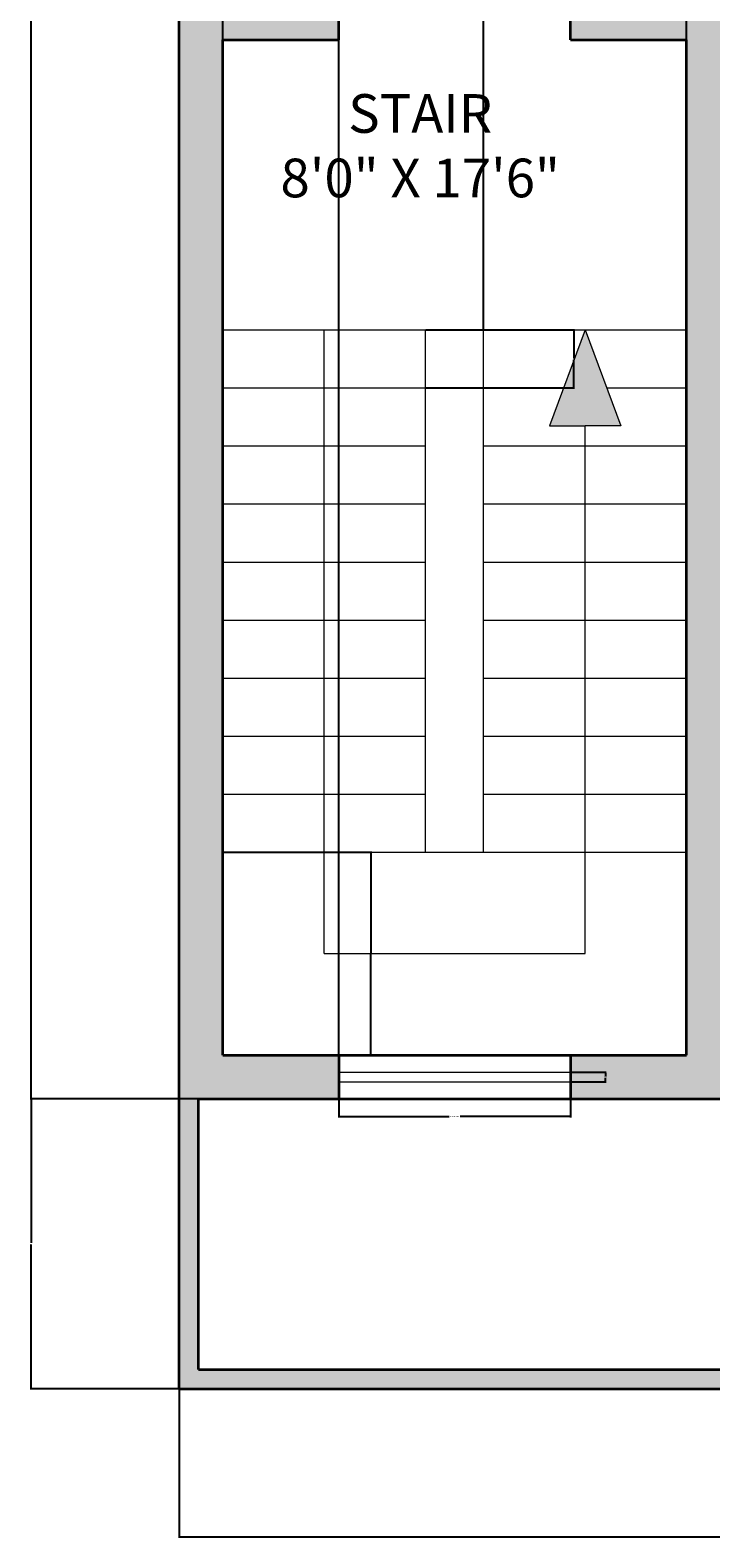
# Model space of a CAD drawing. Units: inches. Extents: x 1567 to 1964, y 1813 to 2447.
# Tile 1 of 28: x 1567 to 1707, y 1813 to 2125. Entities that reach past the tile are written whole.
import ezdxf

# ---------------------------------------------------------------- set-up
doc = ezdxf.new("R2010")
doc.units = ezdxf.units.IN
for name, color, linetype, lineweight in [('A-ANNO-DIMS', 2, 'Continuous', 18), ('A-AREA-IDEN', 7, 'Continuous', 18), ('A-FLOR-STRS', 7, 'Continuous', 18), ('A-GLAZ', 4, 'Continuous', 18), ('A-WALL', 7, 'Continuous', 35)]:
    doc.layers.add(name, color=color, linetype=linetype, lineweight=lineweight)
doc.layers.add('A-FURN-PATT', color=252, linetype='Continuous', lineweight=13, true_color=0x939598)
doc.layers.add('A-WALL-PATT', color=251, linetype='Continuous', lineweight=13, true_color=0x636466)
doc.styles.get("Standard").update_dxf_attribs({"font": 'arial.ttf'})
doc.dimstyles.get("Standard").update_dxf_attribs({"dimtxt": 0.18, "dimasz": 0.18, "dimexe": 0.18, "dimexo": 0.0625, "dimgap": 0.09, "dimtad": 0, "dimtih": 1, "dimtoh": 1, "dimdec": 4, "dimzin": 0, "dimdsep": 46, "dimtxsty": 'Standard', "dimcen": 0.09, "dimadec": 0, "dimazin": 0, "dimtfac": 1, "dimtdec": 4, "dimtofl": 0, "dimtmove": 0, "dimatfit": 3, "dimfxl": 1, "dimtolj": 1, "dimtzin": 0, "dimarcsym": 0})

# ---------------------------------------------------------------- blocks, each defined once
blk = doc.blocks.new('WINDOW-48IN')
for p, q in [((0, 2), (48, 2)), ((0, 0), (48, 0))]:
    blk.add_line(p, q)
blk = doc.blocks.new('*D35')
at = {"layer": 'A-ANNO-DIMS', "color": 0, "lineweight": -2, "transparency": 16777216}
for p, q in [((1630.43, 1907.73), (1630.43, 1900.41)), ((1678.43, 1907.73), (1678.43, 1900.41)), ((1630.61, 1900.59), (1653.31, 1900.59)), ((1678.25, 1900.59), (1655.55, 1900.59))]:
    blk.add_line(p, q, dxfattribs=at)
at = {"layer": 'A-ANNO-DIMS', "color": 0, "transparency": 16777216}
for points in [[(1630.61, 1900.62), (1630.61, 1900.56), (1630.43, 1900.59)], [(1678.25, 1900.62), (1678.25, 1900.56), (1678.43, 1900.59)]]:
    blk.add_solid(points, dxfattribs=at)
at = {"layer": 'Defpoints', "color": 0, "transparency": 16777216}
for p in [(1630.43, 1907.79), (1678.43, 1907.79), (1678.43, 1900.59)]:
    blk.add_point(p, dxfattribs=at)
at = {"layer": 'A-ANNO-DIMS', "color": 0, "transparency": 16777216, "insert": (1654.43, 1900.59), "char_height": 0.18, "attachment_point": 5}
blk.add_mtext('\\A1;WINDOW 48 TYP.', dxfattribs=at)
blk = doc.blocks.new('*D36')
at = {"layer": 'A-ANNO-DIMS', "color": 0, "lineweight": -2, "transparency": 16777216}
for p, q in [((1678.49, 1909.79), (1685.81, 1909.79)), ((1685.63, 1909.61), (1685.63, 1908.97)), ((1685.63, 1907.97), (1685.63, 1908.61)), ((1678.49, 1907.79), (1685.81, 1907.79))]:
    blk.add_line(p, q, dxfattribs=at)
at = {"layer": 'A-ANNO-DIMS', "color": 0, "transparency": 16777216}
for points in [[(1685.6, 1909.61), (1685.66, 1909.61), (1685.63, 1909.79)], [(1685.6, 1907.97), (1685.66, 1907.97), (1685.63, 1907.79)]]:
    blk.add_solid(points, dxfattribs=at)
at = {"layer": 'Defpoints', "color": 0, "transparency": 16777216}
for p in [(1678.43, 1909.79), (1685.63, 1909.79), (1678.43, 1907.79)]:
    blk.add_point(p, dxfattribs=at)
at = {"layer": 'A-ANNO-DIMS', "color": 0, "transparency": 16777216, "insert": (1685.63, 1908.79), "char_height": 0.18, "attachment_point": 5}
blk.add_mtext('\\A1;2 TYP.', dxfattribs=at)
blk = doc.blocks.new('*D39')
at = {"layer": 'A-ANNO-DIMS', "color": 0, "lineweight": -2, "transparency": 16777216}
for p, q in [((1597.43, 1844.23), (1597.43, 1813.46)), ((1933.43, 1844.23), (1933.43, 1813.46)), ((1597.61, 1813.64), (1765.14, 1813.64)), ((1933.25, 1813.64), (1765.72, 1813.64))]:
    blk.add_line(p, q, dxfattribs=at)
at = {"layer": 'A-ANNO-DIMS', "color": 0, "transparency": 16777216}
for points in [[(1597.61, 1813.67), (1597.61, 1813.61), (1597.43, 1813.64)], [(1933.25, 1813.67), (1933.25, 1813.61), (1933.43, 1813.64)]]:
    blk.add_solid(points, dxfattribs=at)
at = {"layer": 'Defpoints', "color": 0, "transparency": 16777216}
for p in [(1597.43, 1844.29), (1933.43, 1844.29), (1933.43, 1813.64)]:
    blk.add_point(p, dxfattribs=at)
at = {"layer": 'A-ANNO-DIMS', "color": 0, "transparency": 16777216, "insert": (1765.43, 1813.64), "char_height": 0.18, "attachment_point": 5}
blk.add_mtext('\\A1;336', dxfattribs=at)
blk = doc.blocks.new('*D41')
at = {"layer": 'A-ANNO-DIMS', "color": 0, "lineweight": -2, "transparency": 16777216}
for p, q in [((1597.37, 2416.29), (1566.6, 2416.29)), ((1566.78, 2416.11), (1566.78, 2160.47)), ((1566.78, 1904.47), (1566.78, 2160.11)), ((1601.37, 1904.29), (1566.6, 1904.29))]:
    blk.add_line(p, q, dxfattribs=at)
at = {"layer": 'A-ANNO-DIMS', "color": 0, "transparency": 16777216}
for points in [[(1566.75, 2416.11), (1566.81, 2416.11), (1566.78, 2416.29)], [(1566.75, 1904.47), (1566.81, 1904.47), (1566.78, 1904.29)]]:
    blk.add_solid(points, dxfattribs=at)
at = {"layer": 'Defpoints', "color": 0, "transparency": 16777216}
for p in [(1566.78, 2416.29), (1597.43, 2416.29), (1601.43, 1904.29)]:
    blk.add_point(p, dxfattribs=at)
at = {"layer": 'A-ANNO-DIMS', "color": 0, "transparency": 16777216, "insert": (1566.78, 2160.29), "char_height": 0.18, "attachment_point": 5}
blk.add_mtext('\\A1;512', dxfattribs=at)
blk = doc.blocks.new('*D42')
at = {"layer": 'A-ANNO-DIMS', "color": 0, "lineweight": -2, "transparency": 16777216}
for p, q in [((1601.37, 1904.29), (1566.6, 1904.29)), ((1566.78, 1904.11), (1566.78, 1874.47)), ((1566.78, 1844.47), (1566.78, 1874.11)), ((1597.37, 1844.29), (1566.6, 1844.29))]:
    blk.add_line(p, q, dxfattribs=at)
at = {"layer": 'A-ANNO-DIMS', "color": 0, "transparency": 16777216}
for points in [[(1566.75, 1904.11), (1566.81, 1904.11), (1566.78, 1904.29)], [(1566.75, 1844.47), (1566.81, 1844.47), (1566.78, 1844.29)]]:
    blk.add_solid(points, dxfattribs=at)
at = {"layer": 'Defpoints', "color": 0, "transparency": 16777216}
for p in [(1566.78, 1904.29), (1601.43, 1904.29), (1597.43, 1844.29)]:
    blk.add_point(p, dxfattribs=at)
at = {"layer": 'A-ANNO-DIMS', "color": 0, "transparency": 16777216, "insert": (1566.78, 1874.29), "char_height": 0.18, "attachment_point": 5}
blk.add_mtext('\\A1;60', dxfattribs=at)
blk = doc.blocks.new('*D53')
at = {"layer": 'A-ANNO-DIMS', "color": 0, "lineweight": -2, "transparency": 16777216}
for p, q in [((1606.43, 1913.35), (1606.43, 2447.12)), ((1606.61, 2446.94), (1618.21, 2446.94)), ((1630.25, 2446.94), (1618.65, 2446.94)), ((1630.43, 1913.35), (1630.43, 2447.12))]:
    blk.add_line(p, q, dxfattribs=at)
at = {"layer": 'A-ANNO-DIMS', "color": 0, "transparency": 16777216}
for points in [[(1606.61, 2446.97), (1606.61, 2446.91), (1606.43, 2446.94)], [(1630.25, 2446.97), (1630.25, 2446.91), (1630.43, 2446.94)]]:
    blk.add_solid(points, dxfattribs=at)
at = {"layer": 'Defpoints', "color": 0, "transparency": 16777216}
for p in [(1630.43, 2446.94), (1606.43, 1913.29), (1630.43, 1913.29)]:
    blk.add_point(p, dxfattribs=at)
at = {"layer": 'A-ANNO-DIMS', "color": 0, "transparency": 16777216, "insert": (1618.43, 2446.94), "char_height": 0.18, "attachment_point": 5}
blk.add_mtext('\\A1;24', dxfattribs=at)
blk = doc.blocks.new('*D60')
at = {"layer": 'A-ANNO-DIMS', "color": 0, "lineweight": -2, "transparency": 16777216}
for p, q in [((1660.43, 2063.35), (1660.43, 2447.12)), ((1660.61, 2446.94), (1681.21, 2446.94)), ((1702.25, 2446.94), (1681.65, 2446.94)), ((1702.43, 2063.35), (1702.43, 2447.12))]:
    blk.add_line(p, q, dxfattribs=at)
at = {"layer": 'A-ANNO-DIMS', "color": 0, "transparency": 16777216}
for points in [[(1660.61, 2446.97), (1660.61, 2446.91), (1660.43, 2446.94)], [(1702.25, 2446.97), (1702.25, 2446.91), (1702.43, 2446.94)]]:
    blk.add_solid(points, dxfattribs=at)
at = {"layer": 'Defpoints', "color": 0, "transparency": 16777216}
for p in [(1660.43, 2446.94), (1660.43, 2063.29), (1702.43, 2063.29)]:
    blk.add_point(p, dxfattribs=at)
at = {"layer": 'A-ANNO-DIMS', "color": 0, "transparency": 16777216, "insert": (1681.43, 2446.94), "char_height": 0.18, "attachment_point": 5}
blk.add_mtext('\\A1;42', dxfattribs=at)
blk = doc.blocks.new('*D61')
at = {"layer": 'A-ANNO-DIMS', "color": 0, "lineweight": -2, "transparency": 16777216}
for p, q in [((1648.49, 2063.29), (1679.26, 2063.29)), ((1679.08, 2063.11), (1679.08, 2057.47)), ((1679.08, 2051.47), (1679.08, 2057.11)), ((1648.49, 2051.29), (1679.26, 2051.29))]:
    blk.add_line(p, q, dxfattribs=at)
at = {"layer": 'A-ANNO-DIMS', "color": 0, "transparency": 16777216}
for points in [[(1679.05, 2063.11), (1679.11, 2063.11), (1679.08, 2063.29)], [(1679.05, 2051.47), (1679.11, 2051.47), (1679.08, 2051.29)]]:
    blk.add_solid(points, dxfattribs=at)
at = {"layer": 'Defpoints', "color": 0, "transparency": 16777216}
for p in [(1648.43, 2063.29), (1648.43, 2051.29), (1679.08, 2051.29)]:
    blk.add_point(p, dxfattribs=at)
at = {"layer": 'A-ANNO-DIMS', "color": 0, "transparency": 16777216, "insert": (1679.08, 2057.29), "char_height": 0.18, "attachment_point": 5}
blk.add_mtext('\\A1;12', dxfattribs=at)
blk = doc.blocks.new('*D62')
at = {"layer": 'A-ANNO-DIMS', "color": 0, "lineweight": -2, "transparency": 16777216}
for p, q in [((1606.49, 1955.29), (1637.26, 1955.29)), ((1637.08, 1955.11), (1637.08, 1934.47)), ((1637.08, 1913.47), (1637.08, 1934.11)), ((1606.49, 1913.29), (1637.26, 1913.29))]:
    blk.add_line(p, q, dxfattribs=at)
at = {"layer": 'A-ANNO-DIMS', "color": 0, "transparency": 16777216}
for points in [[(1637.05, 1955.11), (1637.11, 1955.11), (1637.08, 1955.29)], [(1637.05, 1913.47), (1637.11, 1913.47), (1637.08, 1913.29)]]:
    blk.add_solid(points, dxfattribs=at)
at = {"layer": 'Defpoints', "color": 0, "transparency": 16777216}
for p in [(1606.43, 1955.29), (1606.43, 1913.29), (1637.08, 1913.29)]:
    blk.add_point(p, dxfattribs=at)
at = {"layer": 'A-ANNO-DIMS', "color": 0, "transparency": 16777216, "insert": (1637.08, 1934.29), "char_height": 0.18, "attachment_point": 5}
blk.add_mtext('\\A1;42', dxfattribs=at)

msp = doc.modelspace()

# ---------------------------------------------------------------- hatches: boundary and pattern name
at = {"layer": 'A-FURN-PATT'}
h = msp.add_hatch(color=256, dxfattribs=at)
h.dxf.hatch_style = 1
h.paths.add_polyline_path([(1697.3402, 2374.8316), (1682.1402, 2374.8316), (1682.1402, 2387.6316), (1637.3402, 2387.6316), (1637.3402, 2324.4315), (1697.3402, 2324.4315)])
h.paths.add_polyline_path([(1891.1093, 2375.8204), (1875.9094, 2375.8204), (1875.9094, 2388.6204), (1831.1094, 2388.6204), (1831.1094, 2325.4204), (1891.1093, 2325.4204)])
h.paths.add_polyline_path([(1702.5611, 2206.8057), (1702.5611, 2210.8057), (1699.7395, 2209.9436), (1697.013, 2209.2403), (1694.3857, 2208.6763), (1691.8615, 2208.2326), (1689.4443, 2207.8896), (1687.1381, 2207.6282), (1684.9469, 2207.4289), (1682.8747, 2207.2725), (1680.9233, 2207.1425), (1679.0865, 2207.0339), (1677.3558, 2206.9445), (1675.7229, 2206.8719), (1674.1794, 2206.8141), (1672.7169, 2206.7688), (1671.327, 2206.7339), (1670.0014, 2206.707), (1668.7314, 2206.6866), (1667.5072, 2206.6732), (1666.3188, 2206.668), (1665.1561, 2206.6722), (1664.009, 2206.6869), (1662.8675, 2206.7133), (1661.7215, 2206.7525), (1660.5611, 2206.8057), (1660.5611, 2202.8057), (1661.9932, 2202.9556), (1663.3314, 2203.0744), (1664.5899, 2203.1671), (1665.7831, 2203.2385), (1666.9254, 2203.2935), (1668.0311, 2203.3368), (1669.1145, 2203.3734), (1670.1902, 2203.4081), (1671.2724, 2203.4451), (1672.3759, 2203.4866), (1673.5155, 2203.534), (1674.706, 2203.5887), (1675.9621, 2203.6523), (1677.2986, 2203.7262), (1678.7304, 2203.8118), (1680.2722, 2203.9108), (1681.947, 2204.0272), (1683.8108, 2204.1769), (1685.9279, 2204.3782), (1688.3626, 2204.6496), (1691.179, 2205.0096), (1694.4413, 2205.4767), (1698.214, 2206.0692)])
h.paths.add_polyline_path([(1702.5611, 2218.8057), (1701.9821, 2217.9383), (1701.3316, 2217.191), (1700.6091, 2216.5515), (1699.8141, 2216.0071), (1698.946, 2215.5454), (1698.0041, 2215.1536), (1696.9879, 2214.8194), (1695.8969, 2214.5301), (1694.7328, 2214.2753), (1693.5072, 2214.0522), (1692.2339, 2213.8602), (1690.9266, 2213.6989), (1689.5994, 2213.5675), (1688.266, 2213.4654), (1686.9402, 2213.392), (1685.636, 2213.3467), (1684.3619, 2213.3287), (1683.1053, 2213.3361), (1681.8482, 2213.3668), (1680.5727, 2213.4187), (1679.2608, 2213.4898), (1677.8948, 2213.5779), (1676.4565, 2213.6811), (1674.9282, 2213.7971), (1673.2982, 2213.9236), (1671.5804, 2214.0573), (1669.795, 2214.1945), (1667.9622, 2214.3316), (1666.1022, 2214.4649), (1664.2352, 2214.5908), (1662.3814, 2214.7056), (1660.5611, 2214.8057), (1660.5611, 2206.8057), (1661.7215, 2206.7525), (1662.8675, 2206.7133), (1664.009, 2206.6869), (1665.1561, 2206.6722), (1666.3188, 2206.668), (1667.5072, 2206.6732), (1668.7314, 2206.6866), (1670.0014, 2206.707), (1671.327, 2206.7339), (1672.7169, 2206.7688), (1674.1794, 2206.8141), (1675.7229, 2206.8719), (1677.3558, 2206.9445), (1679.0865, 2207.0339), (1680.9233, 2207.1425), (1682.8747, 2207.2725), (1684.9469, 2207.4289), (1687.1381, 2207.6282), (1689.4443, 2207.8896), (1691.8615, 2208.2326), (1694.3857, 2208.6763), (1697.013, 2209.2403), (1699.7395, 2209.9436), (1702.5611, 2210.8057)])
h.paths.add_polyline_path([(1700.6091, 2216.5515), (1701.3316, 2217.191), (1701.9821, 2217.9383), (1702.5611, 2218.8057), (1702.5611, 2222.8057), (1689.452, 2222.8057), (1689.0171, 2222.4556), (1688.4521, 2222.0354), (1687.7806, 2221.5662), (1687.0235, 2221.067), (1686.2019, 2220.5566), (1685.3367, 2220.0541), (1684.4491, 2219.5785), (1683.56, 2219.1486), (1682.6867, 2218.7795), (1681.8312, 2218.4692), (1680.9918, 2218.212), (1680.1667, 2218.0019), (1679.3541, 2217.833), (1678.5524, 2217.6995), (1677.7597, 2217.5954), (1676.9744, 2217.5149), (1676.1942, 2217.4531), (1675.4146, 2217.4093), (1674.6309, 2217.384), (1673.8381, 2217.3774), (1673.0313, 2217.39), (1672.2056, 2217.4221), (1671.3562, 2217.4741), (1670.4782, 2217.5463), (1669.5642, 2217.639), (1668.5968, 2217.7516), (1667.5562, 2217.8833), (1666.4226, 2218.0336), (1665.1761, 2218.2017), (1663.7969, 2218.3869), (1662.2651, 2218.5885), (1660.5611, 2218.8057), (1660.5611, 2214.8057), (1662.3814, 2214.7056), (1664.2352, 2214.5908), (1666.1022, 2214.4649), (1667.9622, 2214.3316), (1669.795, 2214.1945), (1671.5804, 2214.0573), (1673.2982, 2213.9236), (1674.9282, 2213.7971), (1676.4565, 2213.6811), (1677.8948, 2213.5779), (1679.2608, 2213.4898), (1680.5727, 2213.4187), (1681.8482, 2213.3668), (1683.1053, 2213.3361), (1684.3619, 2213.3287), (1685.636, 2213.3467), (1686.9402, 2213.392), (1688.266, 2213.4654), (1689.5994, 2213.5675), (1690.9266, 2213.6989), (1692.2339, 2213.8602), (1693.5072, 2214.0522), (1694.7328, 2214.2753), (1695.8969, 2214.5301), (1696.9879, 2214.8194), (1698.0041, 2215.1536), (1698.946, 2215.5454), (1699.8141, 2216.0071)])
h.paths.add_polyline_path([(1687.0235, 2221.067), (1687.7806, 2221.5662), (1688.4521, 2222.0354), (1689.0171, 2222.4556), (1689.452, 2222.8057), (1660.5611, 2222.8057), (1660.5611, 2218.8057), (1662.2651, 2218.5885), (1663.7969, 2218.3869), (1665.1761, 2218.2017), (1666.4226, 2218.0336), (1667.5562, 2217.8833), (1668.5968, 2217.7516), (1669.5642, 2217.639), (1670.4782, 2217.5463), (1671.3562, 2217.4741), (1672.2056, 2217.4221), (1673.0313, 2217.39), (1673.8381, 2217.3774), (1674.6309, 2217.384), (1675.4146, 2217.4093), (1676.1942, 2217.4531), (1676.9744, 2217.5149), (1677.7597, 2217.5954), (1678.5524, 2217.6995), (1679.3541, 2217.833), (1680.1667, 2218.0019), (1680.9918, 2218.212), (1681.8312, 2218.4692), (1682.6867, 2218.7795), (1683.56, 2219.1486), (1684.4491, 2219.5785), (1685.3367, 2220.0541), (1686.2019, 2220.5566)], flags=17)
h.paths.add_polyline_path([(1702.5611, 2198.8057), (1698.9289, 2199.2412), (1695.8472, 2199.5774), (1693.2166, 2199.8257), (1690.9377, 2199.9973), (1688.9111, 2200.1033), (1687.0375, 2200.155), (1685.2174, 2200.1637), (1683.3514, 2200.1406), (1681.3514, 2200.0941), (1679.1736, 2200.0225), (1676.7858, 2199.921), (1674.1554, 2199.7852), (1671.2502, 2199.6103), (1668.0377, 2199.3919), (1664.4854, 2199.1252), (1660.5611, 2198.8057), (1660.5611, 2194.8057), (1662.2697, 2194.9771), (1663.9673, 2195.0999), (1665.6339, 2195.1809), (1667.2495, 2195.227), (1668.7941, 2195.2449), (1670.2478, 2195.2414), (1671.5906, 2195.2233), (1672.8026, 2195.1974), (1673.8739, 2195.1689), (1674.8359, 2195.1364), (1675.7302, 2195.0967), (1676.5982, 2195.0469), (1677.4817, 2194.9838), (1678.422, 2194.9043), (1679.4609, 2194.8055), (1680.6397, 2194.6842), (1682.005, 2194.5341), (1683.6223, 2194.335), (1685.562, 2194.0637), (1687.8945, 2193.6967), (1690.6902, 2193.2108), (1694.0196, 2192.5826), (1697.9531, 2191.7887), (1702.5611, 2190.8057)])
h.paths.add_polyline_path([(1702.5611, 2206.8057), (1698.214, 2206.0692), (1694.4413, 2205.4767), (1691.179, 2205.0096), (1688.3626, 2204.6496), (1685.9279, 2204.3782), (1683.8108, 2204.1769), (1681.947, 2204.0272), (1680.2722, 2203.9108), (1678.7304, 2203.8118), (1677.2986, 2203.7262), (1675.9621, 2203.6523), (1674.706, 2203.5887), (1673.5155, 2203.534), (1672.3759, 2203.4866), (1671.2724, 2203.4451), (1670.1902, 2203.4081), (1669.1145, 2203.3734), (1668.0311, 2203.3368), (1666.9254, 2203.2935), (1665.7831, 2203.2385), (1664.5899, 2203.1671), (1663.3314, 2203.0744), (1661.9932, 2202.9556), (1660.5611, 2202.8057), (1660.5611, 2198.8057), (1664.4854, 2199.1252), (1668.0377, 2199.3919), (1671.2502, 2199.6103), (1674.1554, 2199.7852), (1676.7858, 2199.921), (1679.1736, 2200.0225), (1681.3514, 2200.0941), (1683.3514, 2200.1406), (1685.2174, 2200.1637), (1687.0375, 2200.155), (1688.9111, 2200.1033), (1690.9377, 2199.9973), (1693.2166, 2199.8257), (1695.8472, 2199.5774), (1698.9289, 2199.2412), (1702.5611, 2198.8057)])
h.paths.add_polyline_path([(1702.5611, 2190.8057), (1697.9531, 2191.7887), (1694.0196, 2192.5826), (1690.6902, 2193.2108), (1687.8945, 2193.6967), (1685.562, 2194.0637), (1683.6223, 2194.335), (1682.005, 2194.5341), (1680.6397, 2194.6842), (1679.4609, 2194.8055), (1678.422, 2194.9043), (1677.4817, 2194.9838), (1676.5982, 2195.0469), (1675.7302, 2195.0967), (1674.8359, 2195.1364), (1673.8739, 2195.1689), (1672.8026, 2195.1974), (1671.5906, 2195.2233), (1670.2478, 2195.2414), (1668.7941, 2195.2449), (1667.2495, 2195.227), (1665.6339, 2195.1809), (1663.9673, 2195.0999), (1662.2697, 2194.9771), (1660.5611, 2194.8057), (1660.5611, 2190.8057), (1665.9637, 2190.2699), (1670.5105, 2189.7867), (1674.3035, 2189.3504), (1677.4445, 2188.9552), (1680.0354, 2188.5951), (1682.1782, 2188.2644), (1683.9747, 2187.9571), (1685.5268, 2187.6675), (1686.9225, 2187.3901), (1688.1943, 2187.1216), (1689.3606, 2186.859), (1690.4399, 2186.5993), (1691.4508, 2186.3396), (1692.4118, 2186.0769), (1693.3413, 2185.8084), (1694.2579, 2185.531), (1695.1786, 2185.2422), (1696.1142, 2184.9406), (1697.0739, 2184.6252), (1698.0671, 2184.2949), (1699.1032, 2183.9489), (1700.1913, 2183.586), (1701.3408, 2183.2053), (1702.5611, 2182.8057)])
h.paths.add_polyline_path([(1702.5611, 2182.8057), (1701.3408, 2183.2053), (1700.1913, 2183.586), (1699.1032, 2183.9489), (1698.0671, 2184.2949), (1697.0739, 2184.6252), (1696.1142, 2184.9406), (1695.1786, 2185.2422), (1694.2579, 2185.531), (1693.3413, 2185.8084), (1692.4118, 2186.0769), (1691.4508, 2186.3396), (1690.4399, 2186.5993), (1689.3606, 2186.859), (1688.1943, 2187.1216), (1686.9225, 2187.3901), (1685.5268, 2187.6675), (1683.9747, 2187.9571), (1682.1782, 2188.2644), (1680.0354, 2188.5951), (1677.4445, 2188.9552), (1674.3035, 2189.3504), (1670.5105, 2189.7867), (1665.9637, 2190.2699), (1660.5611, 2190.8057), (1660.5611, 2186.8057), (1663.5709, 2186.52), (1666.0965, 2186.2414), (1668.1979, 2185.9698), (1669.9351, 2185.7048), (1671.3681, 2185.446), (1672.5568, 2185.1931), (1673.5613, 2184.9458), (1674.4415, 2184.7037), (1675.2485, 2184.4664), (1675.9976, 2184.2328), (1677.0295, 2183.8907), (1678.2492, 2183.4332), (1679.354, 2182.9669), (1680.4123, 2182.4724), (1681.3757, 2181.9718), (1682.2435, 2181.4594), (1683.1864, 2180.8057), (1702.5611, 2180.8057)])
h.paths.add_polyline_path([(1677.3469, 2183.7716), (1676.6949, 2184.0016), (1675.9976, 2184.2328), (1675.2485, 2184.4664), (1674.4415, 2184.7037), (1673.5613, 2184.9458), (1672.5568, 2185.1931), (1671.3681, 2185.446), (1669.9351, 2185.7048), (1668.1979, 2185.9698), (1666.0965, 2186.2414), (1663.5709, 2186.52), (1660.5611, 2186.8057), (1660.5611, 2180.8057), (1683.1506, 2180.8057), (1682.802, 2181.0722), (1682.4264, 2181.3326), (1682.0201, 2181.5913), (1681.586, 2181.8476), (1681.1268, 2182.1011), (1680.6453, 2182.3513), (1680.1443, 2182.5976), (1679.6266, 2182.8395), (1679.0933, 2183.0769), (1678.5398, 2183.3105), (1677.9598, 2183.5417)], flags=17)
h.paths.add_polyline_path([(1824.4511, 2199.9016), (1824.089, 2199.9302), (1824.0595, 2199.9372), (1824.0397, 2199.9406), (1823.5413, 2200.0576), (1823.4095, 2200.0864), (1823.0664, 2200.1559), (1822.6419, 2200.2361), (1822.1519, 2200.3222), (1821.6126, 2200.4093), (1821.0401, 2200.4925), (1820.4505, 2200.5669), (1819.8599, 2200.6276), (1819.2845, 2200.6697), (1818.7366, 2200.6896), (1818.2141, 2200.688), (1817.7112, 2200.6668), (1817.222, 2200.6281), (1816.7405, 2200.5737), (1816.261, 2200.5057), (1815.7776, 2200.4259), (1815.2845, 2200.3364), (1814.3007, 2200.149), (1813.3315, 2199.9765), (1812.406, 2199.8514), (1811.6868, 2199.7739), (1810.8992, 2199.7121), (1810.0345, 2199.6697), (1809.0854, 2199.6497), (1808.0514, 2199.6502), (1806.9334, 2199.6683), (1805.7324, 2199.701), (1804.4493, 2199.7454), (1803.0852, 2199.7986), (1801.641, 2199.8577), (1800.1178, 2199.9197), (1798.5134, 2199.9818), (1796.8144, 2200.0415), (1795.004, 2200.0962), (1793.0657, 2200.1437), (1790.9828, 2200.1814), (1788.7389, 2200.2068), (1786.3171, 2200.2177), (1783.7011, 2200.2114), (1780.8715, 2200.185), (1777.7988, 2200.1326), (1774.4506, 2200.0481), (1770.7948, 2199.9249), (1766.7992, 2199.7569), (1762.4316, 2199.5376), (1757.6596, 2199.2606), (1752.4511, 2198.9197), (1752.4511, 2193.4197), (1761.2668, 2193.6071), (1768.3671, 2193.7934), (1773.9821, 2193.9778), (1778.3417, 2194.1593), (1781.6759, 2194.3369), (1784.2148, 2194.5096), (1786.1882, 2194.6764), (1787.8261, 2194.8364), (1789.3219, 2194.9887), (1790.7226, 2195.1333), (1792.0383, 2195.27), (1793.2792, 2195.3989), (1794.4557, 2195.52), (1795.5781, 2195.6333), (1796.6564, 2195.7387), (1797.7011, 2195.8364), (1798.7216, 2195.9259), (1799.7245, 2196.0057), (1800.7158, 2196.0737), (1801.7011, 2196.1281), (1802.6865, 2196.1668), (1803.6777, 2196.188), (1804.6806, 2196.1896), (1805.7011, 2196.1697), (1806.7423, 2196.1273), (1807.7962, 2196.0643), (1808.852, 2195.9837), (1809.899, 2195.8885), (1810.9265, 2195.7815), (1811.9238, 2195.6658), (1812.88, 2195.5442), (1813.7845, 2195.4197), (1814.6296, 2195.2948), (1815.4205, 2195.1704), (1816.1656, 2195.0469), (1816.873, 2194.9249), (1817.5511, 2194.8049), (1818.2083, 2194.6873), (1818.8527, 2194.5726), (1819.4928, 2194.4614), (1820.1348, 2194.3554), (1820.7773, 2194.2615), (1821.4169, 2194.1882), (1822.0501, 2194.1437), (1822.6735, 2194.1363), (1823.2838, 2194.1743), (1823.8775, 2194.266), (1824.4511, 2194.4197)])
h.paths.add_polyline_path([(1821.4716, 2190.5098), (1820.4303, 2190.5708), (1819.3811, 2190.6415), (1818.3339, 2190.7186), (1817.2985, 2190.7986), (1816.2845, 2190.8781), (1815.2976, 2190.9542), (1814.3274, 2191.0259), (1813.3592, 2191.0927), (1812.3782, 2191.1541), (1811.3699, 2191.2097), (1810.3196, 2191.2589), (1809.2127, 2191.3013), (1808.0345, 2191.3364), (1806.7708, 2191.3634), (1805.4094, 2191.3807), (1803.9387, 2191.3862), (1802.3469, 2191.3781), (1800.6223, 2191.3543), (1798.7532, 2191.313), (1796.7278, 2191.2521), (1794.5344, 2191.1697), (1792.128, 2191.0648), (1789.33, 2190.9393), (1785.9285, 2190.7962), (1781.7115, 2190.6385), (1776.4672, 2190.469), (1769.9836, 2190.2908), (1762.0489, 2190.1067), (1752.4511, 2189.9197), (1752.4511, 2185.4197), (1758.363, 2185.5846), (1763.4179, 2185.7075), (1767.7199, 2185.7933), (1771.373, 2185.8468), (1774.4811, 2185.873), (1777.1484, 2185.8768), (1779.4787, 2185.8629), (1781.5761, 2185.8364), (1783.5287, 2185.8014), (1785.3606, 2185.7596), (1787.0802, 2185.7119), (1788.6959, 2185.6593), (1790.2158, 2185.6028), (1791.6484, 2185.5434), (1793.0018, 2185.4821), (1794.2844, 2185.4197), (1795.5065, 2185.3576), (1796.6861, 2185.298), (1797.8433, 2185.2432), (1798.998, 2185.1958), (1800.1703, 2185.1581), (1801.3801, 2185.1326), (1802.6476, 2185.1218), (1803.9928, 2185.1281), (1805.4444, 2185.1555), (1807.0663, 2185.2147), (1808.9315, 2185.3178), (1811.1126, 2185.477), (1813.6823, 2185.7046), (1816.7135, 2186.0128), (1820.2788, 2186.4138), (1824.4511, 2186.9197), (1824.4511, 2190.4197), (1823.4918, 2190.4309), (1822.4954, 2190.4621)])
h.paths.add_polyline_path([(1797.3762, 2216.0584), (1797.6199, 2216.2267), (1797.9558, 2216.3355), (1798.3017, 2216.3703), (1798.5761, 2216.3781), (1798.8974, 2216.3703), (1799.2714, 2216.3468), (1799.704, 2216.3078), (1800.2011, 2216.2531), (1800.7695, 2216.1829), (1801.4205, 2216.0981), (1802.1662, 2215.9996), (1803.0188, 2215.8885), (1803.9906, 2215.7656), (1805.0937, 2215.632), (1806.3404, 2215.4886), (1807.7428, 2215.3364), (1809.3101, 2215.1764), (1811.039, 2215.0096), (1812.9232, 2214.8369), (1814.9563, 2214.6593), (1817.132, 2214.4778), (1819.444, 2214.2934), (1821.8858, 2214.1071), (1824.4511, 2213.9197), (1824.4511, 2217.9197), (1752.4511, 2217.9197), (1752.4511, 2214.9197), (1757.2739, 2214.8973), (1761.6432, 2214.8338), (1765.5973, 2214.7352), (1769.1751, 2214.6072), (1772.4149, 2214.4559), (1775.3554, 2214.2869), (1778.0352, 2214.1063), (1780.4928, 2213.9197), (1782.7607, 2213.7329), (1784.8476, 2213.5499), (1786.7557, 2213.3748), (1788.4876, 2213.2114), (1790.0456, 2213.0636), (1791.4322, 2212.9354), (1792.6499, 2212.8305), (1793.7011, 2212.7531), (1794.5904, 2212.7059), (1795.3313, 2212.688), (1795.9394, 2212.6974), (1796.4303, 2212.7322), (1796.8196, 2212.7905), (1797.123, 2212.8703), (1797.356, 2212.9695), (1797.5344, 2213.0864), (1797.6716, 2213.2187), (1797.7727, 2213.3637), (1797.8406, 2213.5185), (1797.8782, 2213.6801), (1797.8884, 2213.8457), (1797.8743, 2214.0122), (1797.8386, 2214.1767), (1797.7844, 2214.3364), (1797.7149, 2214.4889), (1797.6347, 2214.6346), (1797.5486, 2214.7744), (1797.3327, 2215.109), (1797.178, 2215.4303), (1797.1896, 2215.7939)])
h.paths.add_polyline_path([(1804.7872, 2210.6789), (1804.546, 2211.022), (1804.3512, 2211.3917), (1804.2466, 2211.7546), (1804.2574, 2212.0998), (1804.4058, 2212.4178), (1804.7068, 2212.7007), (1805.1359, 2212.9124), (1805.5279, 2212.9926), (1805.8136, 2213.0154), (1806.1178, 2213.0031), (1806.4405, 2212.9529), (1806.7929, 2212.867), (1807.1893, 2212.7489), (1807.6438, 2212.602), (1808.1706, 2212.4297), (1808.7838, 2212.2355), (1809.4976, 2212.0227), (1810.3261, 2211.7947), (1811.2868, 2211.5533), (1812.4101, 2211.2928), (1813.7297, 2211.0059), (1815.2793, 2210.6854), (1817.0925, 2210.3238), (1819.2031, 2209.9139), (1821.6447, 2209.4483), (1824.4511, 2208.9197), (1824.4511, 2213.9197), (1821.8858, 2214.1071), (1819.444, 2214.2934), (1817.132, 2214.4778), (1814.9563, 2214.6593), (1812.9232, 2214.8369), (1811.039, 2215.0096), (1809.3101, 2215.1764), (1807.7428, 2215.3364), (1806.3404, 2215.4886), (1805.0937, 2215.632), (1803.9906, 2215.7656), (1803.0188, 2215.8885), (1802.1662, 2215.9996), (1801.4205, 2216.0981), (1800.7695, 2216.1829), (1800.2011, 2216.2531), (1799.704, 2216.3078), (1799.2714, 2216.3468), (1798.8974, 2216.3703), (1798.5761, 2216.3781), (1798.3017, 2216.3703), (1798.0683, 2216.3468), (1797.87, 2216.3078), (1797.7011, 2216.2531), (1797.5566, 2216.1831), (1797.4355, 2216.0994), (1797.3378, 2216.004), (1797.2636, 2215.8989), (1797.2128, 2215.7859), (1797.1855, 2215.6671), (1797.1816, 2215.5444), (1797.2011, 2215.4197), (1797.2433, 2215.2946), (1797.304, 2215.1684), (1797.3783, 2215.0403), (1797.4615, 2214.9093), (1797.6718, 2214.5836), (1797.8218, 2214.2545), (1797.8933, 2213.9247), (1797.8728, 2213.5918), (1797.7366, 2213.2814), (1797.4586, 2213.0132), (1797.123, 2212.8703), (1796.8196, 2212.7905), (1796.4303, 2212.7322), (1795.9394, 2212.6974), (1795.3313, 2212.688), (1794.5904, 2212.7059), (1793.7011, 2212.7531), (1792.6499, 2212.8305), (1791.4322, 2212.9354), (1790.0456, 2213.0636), (1788.4876, 2213.2114), (1786.7557, 2213.3748), (1784.8476, 2213.5499), (1782.7607, 2213.7329), (1780.4928, 2213.9197), (1778.0352, 2214.1063), (1775.3554, 2214.2869), (1772.4149, 2214.4559), (1769.1751, 2214.6072), (1765.5973, 2214.7352), (1761.6432, 2214.8338), (1757.2739, 2214.8973), (1752.4511, 2214.9197), (1752.4511, 2209.9197), (1759.4745, 2210.0625), (1765.2786, 2210.1242), (1770.027, 2210.1175), (1773.8834, 2210.0551), (1777.0112, 2209.9498), (1779.5741, 2209.8143), (1781.7357, 2209.6611), (1783.6594, 2209.5031), (1785.4813, 2209.3506), (1787.2265, 2209.2049), (1788.8926, 2209.0651), (1790.4771, 2208.9301), (1791.9777, 2208.7991), (1793.3919, 2208.671), (1794.7171, 2208.5449), (1795.9511, 2208.4197), (1797.0922, 2208.2952), (1798.1425, 2208.1736), (1799.1049, 2208.0579), (1799.9823, 2207.951), (1800.7778, 2207.8558), (1801.4941, 2207.7752), (1802.1342, 2207.7122), (1802.7011, 2207.6697), (1803.1982, 2207.65), (1803.6308, 2207.6528), (1804.0048, 2207.6771), (1804.3261, 2207.7218), (1804.6005, 2207.7861), (1804.8339, 2207.869), (1805.0322, 2207.9694), (1805.2011, 2208.0864), (1805.3455, 2208.2189), (1805.4654, 2208.365), (1805.56, 2208.5229), (1805.6282, 2208.6906), (1805.6691, 2208.866), (1805.6816, 2209.0473), (1805.6648, 2209.2326), (1805.6178, 2209.4197), (1805.5406, 2209.6072), (1805.4381, 2209.7947), (1805.316, 2209.9822), (1805.1803, 2210.1697), (1805.0367, 2210.3572)])
h.paths.add_polyline_path([(1801.4941, 2207.7752), (1800.7778, 2207.8558), (1799.9823, 2207.951), (1799.1049, 2208.0579), (1798.1425, 2208.1736), (1797.0922, 2208.2952), (1795.9511, 2208.4197), (1794.7171, 2208.5449), (1793.3919, 2208.671), (1791.9777, 2208.7991), (1790.4771, 2208.9301), (1788.8926, 2209.0651), (1787.2265, 2209.2049), (1785.4813, 2209.3506), (1783.6594, 2209.5031), (1781.7357, 2209.6611), (1779.5741, 2209.8143), (1777.0112, 2209.9498), (1773.8834, 2210.0551), (1770.027, 2210.1175), (1765.2786, 2210.1242), (1759.4745, 2210.0625), (1752.4511, 2209.9197), (1752.4511, 2205.4197), (1757.7354, 2205.2545), (1762.3821, 2205.1294), (1766.4565, 2205.0374), (1770.024, 2204.9718), (1773.1502, 2204.9258), (1775.9003, 2204.8924), (1778.3399, 2204.8649), (1780.5344, 2204.8364), (1782.5421, 2204.8014), (1784.3925, 2204.7596), (1786.1082, 2204.7119), (1787.7115, 2204.6593), (1789.225, 2204.6028), (1790.6711, 2204.5434), (1792.0724, 2204.4821), (1793.4511, 2204.4197), (1794.8241, 2204.3576), (1796.1855, 2204.2973), (1797.5234, 2204.241), (1798.8261, 2204.1906), (1800.082, 2204.1479), (1801.2792, 2204.115), (1802.4062, 2204.0939), (1803.4511, 2204.0864), (1804.4051, 2204.0942), (1805.2701, 2204.1176), (1806.0512, 2204.1567), (1806.7532, 2204.2114), (1807.381, 2204.2817), (1807.9394, 2204.3676), (1808.4334, 2204.4692), (1808.8678, 2204.5864), (1809.248, 2204.7187), (1809.5813, 2204.8637), (1809.8756, 2205.0185), (1810.1386, 2205.1801), (1810.3782, 2205.3457), (1810.6022, 2205.5122), (1810.9725, 2205.7941), (1811.3803, 2206.072), (1811.739, 2206.2612), (1812.0032, 2206.3781), (1812.2869, 2206.4793), (1812.5931, 2206.563), (1812.9246, 2206.6271), (1813.2845, 2206.6697), (1813.6746, 2206.6894), (1814.0931, 2206.6867), (1814.5369, 2206.6624), (1815.0032, 2206.6176), (1815.489, 2206.5534), (1815.9915, 2206.4705), (1816.5076, 2206.3701), (1817.0345, 2206.2531), (1817.5753, 2206.1196), (1818.1582, 2205.9666), (1818.8172, 2205.7902), (1819.5865, 2205.5864), (1820.5004, 2205.3514), (1821.5931, 2205.0812), (1822.8986, 2204.7719), (1824.4511, 2204.4197), (1824.4511, 2208.9197), (1821.6447, 2209.4483), (1819.2031, 2209.9139), (1817.0925, 2210.3238), (1815.2793, 2210.6854), (1813.7297, 2211.0059), (1812.4101, 2211.2928), (1811.2868, 2211.5533), (1810.3261, 2211.7947), (1809.4976, 2212.0227), (1808.7838, 2212.2355), (1808.1706, 2212.4297), (1807.6438, 2212.602), (1807.1893, 2212.7489), (1806.7929, 2212.867), (1806.4405, 2212.9529), (1806.1178, 2213.0031), (1805.8136, 2213.0154), (1805.5279, 2212.9926), (1805.2638, 2212.9386), (1805.024, 2212.8572), (1804.8116, 2212.7524), (1804.6295, 2212.6281), (1804.4806, 2212.4881), (1804.3678, 2212.3364), (1804.2931, 2212.1764), (1804.2545, 2212.0096), (1804.2491, 2211.8369), (1804.274, 2211.6593), (1804.3263, 2211.4778), (1804.4029, 2211.2934), (1804.5011, 2211.1071), (1804.6178, 2210.9197), (1804.7496, 2210.7322), (1804.8912, 2210.5447), (1805.154, 2210.2061), (1805.3962, 2209.8715), (1805.5964, 2209.5053), (1805.688, 2209.1402), (1805.6629, 2208.7758), (1805.5257, 2208.4385), (1805.2839, 2208.1437), (1804.9434, 2207.9078), (1804.6005, 2207.7861), (1804.3261, 2207.7218), (1804.0048, 2207.6771), (1803.6308, 2207.6528), (1803.1982, 2207.65), (1802.7011, 2207.6697), (1802.1342, 2207.7122)])
h.paths.add_polyline_path([(1824.4511, 2204.4197), (1822.8986, 2204.7719), (1821.5931, 2205.0812), (1820.5004, 2205.3514), (1819.5865, 2205.5864), (1818.8172, 2205.7902), (1818.1582, 2205.9666), (1817.5753, 2206.1196), (1817.0345, 2206.2531), (1816.5076, 2206.3701), (1815.9915, 2206.4705), (1815.489, 2206.5534), (1815.0032, 2206.6176), (1814.5369, 2206.6624), (1814.0931, 2206.6867), (1813.6746, 2206.6894), (1813.2845, 2206.6697), (1812.9246, 2206.6271), (1812.5931, 2206.563), (1812.2869, 2206.4793), (1812.0032, 2206.3781), (1811.739, 2206.2612), (1811.4915, 2206.1307), (1811.2576, 2205.9884), (1811.0345, 2205.8364), (1810.8183, 2205.6767), (1810.4357, 2205.3854), (1810.1386, 2205.1801), (1809.8756, 2205.0185), (1809.5813, 2204.8637), (1809.248, 2204.7187), (1808.8678, 2204.5864), (1808.4334, 2204.4692), (1807.9394, 2204.3676), (1807.381, 2204.2817), (1806.7532, 2204.2114), (1806.0512, 2204.1567), (1805.2701, 2204.1176), (1804.4051, 2204.0942), (1803.4511, 2204.0864), (1802.4062, 2204.0939), (1801.2792, 2204.115), (1800.082, 2204.1479), (1798.8261, 2204.1906), (1797.5234, 2204.241), (1796.1855, 2204.2973), (1794.8241, 2204.3576), (1793.4511, 2204.4197), (1792.0724, 2204.4821), (1790.6711, 2204.5434), (1789.225, 2204.6028), (1787.7115, 2204.6593), (1786.1082, 2204.7119), (1784.3925, 2204.7596), (1782.5421, 2204.8014), (1780.5344, 2204.8364), (1778.3399, 2204.8649), (1775.9003, 2204.8924), (1773.1502, 2204.9258), (1770.024, 2204.9718), (1766.4565, 2205.0374), (1762.3821, 2205.1294), (1757.7354, 2205.2545), (1752.4511, 2205.4197), (1752.4511, 2198.9197), (1757.6596, 2199.2606), (1762.4316, 2199.5376), (1766.7992, 2199.7569), (1770.7948, 2199.9249), (1774.4506, 2200.0481), (1777.7988, 2200.1326), (1780.8715, 2200.185), (1783.7011, 2200.2114), (1786.3171, 2200.2177), (1788.7389, 2200.2068), (1790.9828, 2200.1814), (1793.0657, 2200.1437), (1795.004, 2200.0962), (1796.8144, 2200.0415), (1798.5134, 2199.9818), (1800.1178, 2199.9197), (1801.641, 2199.8577), (1803.0852, 2199.7986), (1804.4493, 2199.7454), (1805.7324, 2199.701), (1806.9334, 2199.6683), (1808.0514, 2199.6502), (1809.0854, 2199.6497), (1810.0345, 2199.6697), (1810.8992, 2199.7121), (1811.6868, 2199.7739), (1812.406, 2199.8514), (1813.0657, 2199.9406), (1813.6746, 2200.0376), (1814.2415, 2200.1385), (1814.7752, 2200.2394), (1815.2845, 2200.3364), (1815.7776, 2200.4259), (1816.261, 2200.5057), (1816.7405, 2200.5737), (1817.222, 2200.6281), (1817.7112, 2200.6668), (1818.2141, 2200.688), (1818.7366, 2200.6896), (1819.2845, 2200.6697), (1819.8599, 2200.6276), (1820.4505, 2200.5669), (1821.0401, 2200.4925), (1821.6126, 2200.4093), (1822.1519, 2200.3222), (1822.6419, 2200.2361), (1823.0664, 2200.1559), (1823.5408, 2200.0598), (1824.0595, 2199.9372), (1824.1105, 2199.9285), (1824.1888, 2199.9223), (1824.2953, 2199.9201), (1824.4511, 2199.9197)])
h.paths.add_polyline_path([(1795.4295, 2021.5492), (1771.4295, 2021.5492), (1771.4295, 1988.29), (1735.4295, 1988.29), (1735.4295, 2055.79), (1711.4295, 2055.79), (1711.4295, 1964.29), (1795.4295, 1964.29)])
h.paths.add_polyline_path([(1681.4295, 2063.29), (1674.0411, 2043.4455), (1681.4295, 2043.4455), (1688.818, 2043.4455)])
h.paths.add_polyline_path([(1843.2327, 2065.967), (1919.26, 2065.967), (1919.26, 2095.8187), (1843.2327, 2095.8187)], flags=9)
at = {"layer": 'A-WALL-PATT'}
h = msp.add_hatch(color=256, dxfattribs=at)
h.dxf.hatch_style = 1
h.paths.add_polyline_path([(1606.4295, 2407.29), (1654.4295, 2407.29), (1654.4295, 2416.29), (1597.4295, 2416.29), (1597.4295, 2217.29), (1606.4295, 2217.29), (1606.4295, 2259.29), (1738.4295, 2259.29), (1738.4295, 2247.29), (1742.4295, 2247.29), (1742.4295, 2259.29), (1742.4295, 2272.29), (1738.4295, 2272.29), (1738.4295, 2263.29), (1606.4295, 2263.29)])
h.paths.add_polyline_path([(1753.4295, 2416.29), (1690.4295, 2416.29), (1690.4295, 2407.29), (1738.4295, 2407.29), (1738.4295, 2308.29), (1742.4295, 2308.29), (1742.4295, 2331.29), (1746.9295, 2331.29), (1746.9295, 2335.29), (1742.4295, 2335.29), (1742.4295, 2407.29), (1753.4295, 2407.29)])
h.paths.add_polyline_path([(1840.4295, 2416.29), (1777.4295, 2416.29), (1777.4295, 2407.29), (1788.4295, 2407.29), (1788.4295, 2335.29), (1776.9295, 2335.29), (1776.9295, 2331.29), (1788.4295, 2331.29), (1788.4295, 2308.29), (1792.4295, 2308.29), (1792.4295, 2407.29), (1840.4295, 2407.29)])
h.paths.add_polyline_path([(1933.4295, 2416.29), (1876.4295, 2416.29), (1876.4295, 2407.29), (1924.4295, 2407.29), (1924.4295, 2263.29), (1792.4295, 2263.29), (1792.4295, 2272.29), (1788.4295, 2272.29), (1788.4295, 2259.29), (1872.4295, 2259.29), (1872.4295, 2171.29), (1880.9295, 2171.29), (1880.9295, 2175.29), (1876.4295, 2175.29), (1876.4295, 2259.29), (1924.4295, 2259.29), (1924.4295, 2229.29), (1933.4295, 2229.29)])
h.paths.add_polyline_path([(1933.4295, 2205.29), (1924.4295, 2205.29), (1924.4295, 2175.29), (1910.9295, 2175.29), (1910.9295, 2171.29), (1924.4295, 2171.29), (1924.4295, 2127.29), (1844.4295, 2127.29), (1844.4295, 2123.29), (1924.4295, 2123.29), (1924.4295, 2063.29), (1933.4295, 2063.29)])
h.paths.add_polyline_path([(1799.4295, 2123.29), (1808.4295, 2123.29), (1808.4295, 2127.29), (1781.4295, 2127.29), (1781.4295, 2123.29), (1795.4295, 2123.29), (1795.4295, 1964.29), (1711.4295, 1964.29), (1711.4295, 2123.29), (1751.4295, 2123.29), (1751.4295, 2127.29), (1742.4295, 2127.29), (1742.4295, 2139.29), (1738.4295, 2139.29), (1738.4295, 2127.29), (1678.4295, 2127.29), (1678.4295, 2123.29), (1702.4295, 2123.29), (1702.4295, 1913.29), (1678.4295, 1913.29), (1678.4295, 1904.29), (1711.4295, 1904.29), (1711.4295, 1960.29), (1795.4295, 1960.29), (1795.4295, 1906.69), (1929.4295, 1906.69), (1929.4295, 1848.29), (1601.4295, 1848.29), (1601.4295, 1904.29), (1630.4295, 1904.29), (1630.4295, 1913.29), (1606.4295, 1913.29), (1606.4295, 2123.29), (1630.4295, 2123.29), (1630.4295, 2127.29), (1606.4295, 2127.29), (1606.4295, 2169.29), (1597.4295, 2169.29), (1597.4295, 1844.29), (1933.4295, 1844.29), (1933.4295, 2027.29), (1924.4295, 2027.29), (1924.4295, 1967.29), (1833.9295, 1967.29), (1833.9295, 1963.29), (1924.4295, 1963.29), (1924.4295, 1910.69), (1799.4295, 1910.69), (1799.4295, 1963.29), (1803.9295, 1963.29), (1803.9295, 1967.29), (1799.4295, 1967.29)])

# ---------------------------------------------------------------- linework, layer by layer
at = {"layer": 'A-FLOR-STRS'}
for p, q in [((1606.4295, 2063.29), (1702.4295, 2063.29)), ((1627.4295, 1934.29), (1627.4295, 2063.29)), ((1648.4295, 1955.29), (1648.4295, 2063.29)), ((1660.4295, 1955.29), (1660.4295, 2063.29)), ((1681.4295, 2063.29), (1674.0411, 2043.4455)), ((1681.4295, 2063.29), (1688.818, 2043.4455)), ((1606.4295, 2051.29), (1648.4295, 2051.29)), ((1660.4295, 2051.29), (1676.9617, 2051.29)), ((1685.8973, 2051.29), (1702.4295, 2051.29)), ((1674.0411, 2043.4455), (1681.4295, 2043.4455)), ((1681.4295, 1934.29), (1681.4295, 2043.4455)), ((1688.818, 2043.4455), (1681.4295, 2043.4455)), ((1606.4295, 2039.29), (1648.4295, 2039.29)), ((1660.4295, 2039.29), (1702.4295, 2039.29)), ((1606.4295, 2027.29), (1648.4295, 2027.29)), ((1660.4295, 2027.29), (1702.4295, 2027.29)), ((1606.4295, 2015.29), (1648.4295, 2015.29)), ((1660.4295, 2015.29), (1702.4295, 2015.29)), ((1606.4295, 2003.29), (1648.4295, 2003.29)), ((1660.4295, 2003.29), (1702.4295, 2003.29)), ((1606.4295, 1991.29), (1648.4295, 1991.29)), ((1660.4295, 1991.29), (1702.4295, 1991.29)), ((1606.4295, 1979.29), (1648.4295, 1979.29)), ((1660.4295, 1979.29), (1702.4295, 1979.29)), ((1606.4295, 1967.29), (1648.4295, 1967.29)), ((1660.4295, 1967.29), (1702.4295, 1967.29)), ((1606.4295, 1955.29), (1702.4295, 1955.29)), ((1627.4295, 1934.29), (1681.4295, 1934.29))]:
    msp.add_line(p, q, dxfattribs=at)
at = {"layer": 'A-WALL'}
for p, q in [((1597.4295, 1844.29), (1597.4295, 2416.29)), ((1630.4295, 2123.29), (1630.4295, 2127.29)), ((1678.4295, 2123.29), (1678.4295, 2127.29)), ((1606.4295, 2123.29), (1630.4295, 2123.29)), ((1606.4295, 1913.29), (1606.4295, 2123.29)), ((1678.4295, 2123.29), (1702.4295, 2123.29)), ((1702.4295, 1913.29), (1702.4295, 2123.29)), ((1606.4295, 1913.29), (1702.4295, 1913.29)), ((1630.4295, 1913.29), (1630.4295, 1904.29)), ((1678.4295, 1913.29), (1678.4295, 1904.29)), ((1601.4295, 1904.29), (1711.4295, 1904.29)), ((1601.4295, 1848.29), (1601.4295, 1904.29)), ((1601.4295, 1848.29), (1929.4295, 1848.29)), ((1597.4295, 1844.29), (1933.4295, 1844.29))]:
    msp.add_line(p, q, dxfattribs=at)

# ---------------------------------------------------------------- block references
at = {"layer": 'A-GLAZ'}
msp.add_blockref('WINDOW-48IN', (1630.43, 1907.79), dxfattribs=at)

# ---------------------------------------------------------------- texts
at = {"layer": 'A-AREA-IDEN', "insert": (1606.4295, 2112.0543), "char_height": 8, "attachment_point": 1}
msp.add_mtext_dynamic_manual_height_columns('\\pxqc;STAIR\\P8\'0" X 17\'6"', width=81.753814, gutter_width=12.5, heights=[0], dxfattribs=at)

# ---------------------------------------------------------------- dimensions: what is measured, and where the dimension line sits
at = {"layer": 'A-ANNO-DIMS'}
for base, p1, p2, picture, middle in [((1630.4295, 2446.94), (1606.4295, 1913.29), (1630.4295, 1913.29), '*D53', (1618.4295, 2446.94)), ((1660.4295, 2446.94), (1702.4295, 2063.29), (1660.4295, 2063.29), '*D60', (1681.4295, 2446.94)), ((1933.4295, 1813.64), (1597.4295, 1844.29), (1933.4295, 1844.29), '*D39', (1765.4295, 1813.64))]:
    dim = msp.add_linear_dim(base=base, p1=p1, p2=p2, dimstyle='Standard', override={"dimdec": 0, "dimlfac": 1, "dimrnd": 0, "dimzin": 0, "dimdsep": 46, "dimlunit": 2}, dxfattribs=at)
    dim.commit()
    dim.dimension.update_dxf_attribs({"geometry": picture, "text_midpoint": middle})
for base, p1, p2, angle, picture, middle in [((1566.7795, 2416.29), (1601.4295, 1904.29), (1597.4295, 2416.29), 90, '*D41', (1566.7795, 2160.29)), ((1679.0795, 2051.29), (1648.4295, 2063.29), (1648.4295, 2051.29), 270, '*D61', (1679.0795, 2057.29)), ((1637.0795, 1913.29), (1606.4295, 1955.29), (1606.4295, 1913.29), 270, '*D62', (1637.0795, 1934.29)), ((1566.7795, 1904.29), (1597.4295, 1844.29), (1601.4295, 1904.29), 90, '*D42', (1566.7795, 1874.29))]:
    dim = msp.add_linear_dim(base=base, p1=p1, p2=p2, angle=angle, dimstyle='Standard', override={"dimdec": 0, "dimlfac": 1, "dimrnd": 0, "dimzin": 0, "dimdsep": 46, "dimlunit": 2}, dxfattribs=at)
    dim.commit()
    dim.dimension.update_dxf_attribs({"geometry": picture, "text_midpoint": middle})
dim = msp.add_linear_dim(base=(1685.6295, 1909.79), p1=(1678.4295, 1907.79), p2=(1678.4295, 1909.79), angle=90, text='<> TYP.', dimstyle='Standard', override={"dimdec": 0, "dimlfac": 1, "dimrnd": 0, "dimzin": 0, "dimdsep": 46, "dimlunit": 2}, dxfattribs=at)
dim.commit()
dim.dimension.update_dxf_attribs({"geometry": '*D36', "text_midpoint": (1685.6295, 1908.79)})
dim = msp.add_linear_dim(base=(1678.4295, 1900.59), p1=(1630.4295, 1907.79), p2=(1678.4295, 1907.79), text='WINDOW <> TYP.', dimstyle='Standard', override={"dimdec": 0, "dimlfac": 1, "dimrnd": 0, "dimzin": 0, "dimdsep": 46, "dimlunit": 2}, dxfattribs=at)
dim.commit()
dim.dimension.update_dxf_attribs({"geometry": '*D35', "text_midpoint": (1654.4295, 1900.59)})

doc.saveas('drawing.dxf')
